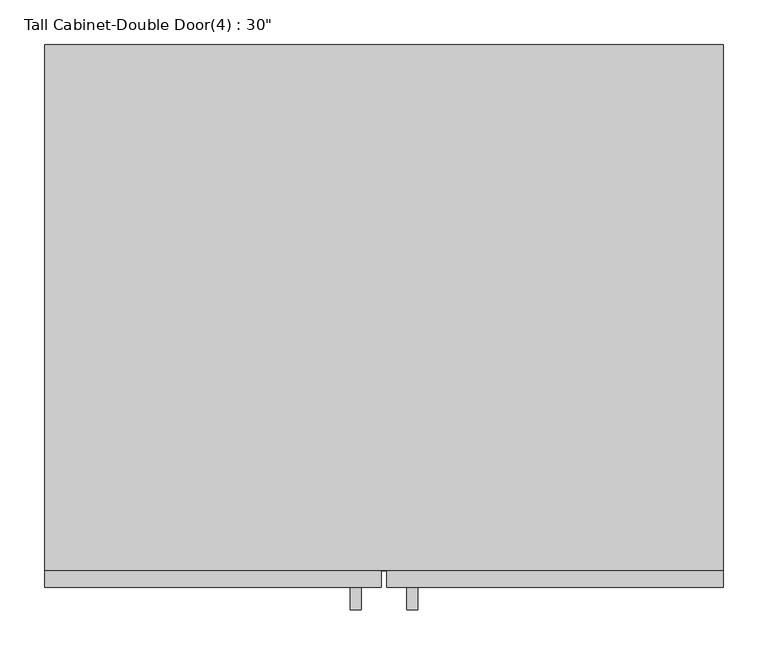
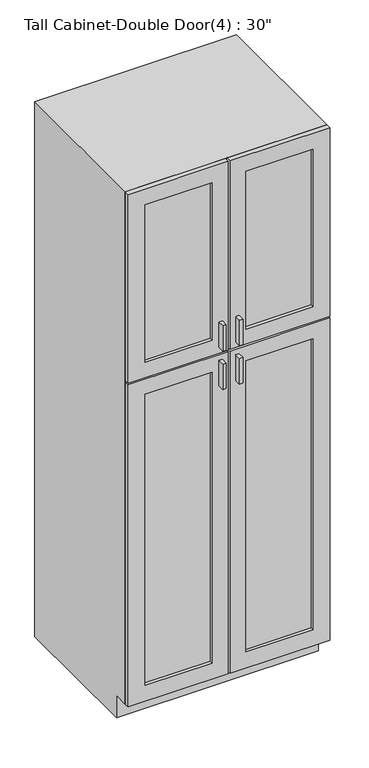
"""IFC4 building model written with IfcOpenShell, lengths in millimetres: furniture geometry."""

from ifc_helpers import new_model, si_unit, frame, origin, place, context, project, spatial, polyline, outline, extrude, faceted_brep, source, transform, mapped, element, save


def furniture_2e4292c0(model_context):
    return source(origin(), model_context, "Body", "SolidModel", [
        faceted_brep([(399.7377049, -590.55, 90.4875), (399.7377049, -590.55, 2133.6), (-362.2622951, -590.55, 2133.6), (-362.2622951, -590.55, 90.4875), (380.6877049, -590.55, 2114.55), (380.6877049, -590.55, 109.5375), (-343.2122951, -590.55, 109.5375), (-343.2122951, -590.55, 2114.55), (-362.2622951, 0.0, 2133.6), (399.7377049, 0.0, 2133.6), (399.7377049, 0.0, 1.5875), (-362.2622951, 0.0, 1.5875), (380.6877049, 0.0, 2114.55), (-343.2122951, 0.0, 2114.55), (-343.2122951, 0.0, 109.5375), (380.6877049, 0.0, 109.5375), (399.7377049, -533.4, 90.4875), (399.7377049, -533.4, 1.5875), (-362.2622951, -533.4, 1.5875), (-362.2622951, -533.4, 90.4875)], [[[0, 1, 2, 3], [4, 5, 6, 7]], [[8, 9, 10, 11], [12, 13, 14, 15]], [[1, 0, 16, 17, 10, 9]], [[2, 1, 9, 8]], [[3, 2, 8, 11, 18, 19]], [[0, 3, 19, 16]], [[5, 4, 12, 15]], [[6, 5, 15, 14]], [[7, 6, 14, 13]], [[4, 7, 13, 12]], [[10, 17, 18, 11]], [[18, 17, 16, 19]]]),
        extrude(outline(polyline([(-6.6622951, -635.0), (-19.1945267, -635.0), (-19.1945267, -609.6), (-6.6622951, -609.6), (-6.6622951, -635.0)])), frame((0.0, 0.0, 1403.5480367), z_axis=(0.0, 0.0, 1.0), x_axis=(1.0, 0.0, 0.0)), (0.0, 0.0, 1.0), 101.6),
        extrude(outline(polyline([(56.6699365, -635.0), (44.1377049, -635.0), (44.1377049, -609.6), (56.6699365, -609.6), (56.6699365, -635.0)])), frame((0.0, 0.0, 1403.5480367), z_axis=(0.0, 0.0, 1.0), x_axis=(1.0, 0.0, 0.0)), (0.0, 0.0, 1.0), 101.6),
        extrude(outline(polyline([(-6.6622951, -635.0), (-19.1945267, -635.0), (-19.1945267, -609.6), (-6.6622951, -609.6), (-6.6622951, -635.0)])), frame((0.0, 0.0, 1251.1480367), z_axis=(0.0, 0.0, 1.0), x_axis=(1.0, 0.0, 0.0)), (0.0, 0.0, 1.0), 101.6),
        extrude(outline(polyline([(56.6699365, -635.0), (44.1377049, -635.0), (44.1377049, -609.6), (56.6699365, -609.6), (56.6699365, -635.0)])), frame((0.0, 0.0, 1251.1480367), z_axis=(0.0, 0.0, 1.0), x_axis=(1.0, 0.0, 0.0)), (0.0, 0.0, 1.0), 101.6),
        extrude(outline(polyline([(-44.7622951, -596.9), (-298.7622951, -596.9), (-298.7622951, -590.55), (-44.7622951, -590.55), (-44.7622951, -596.9)])), frame((0.0, 0.0, 1441.6480367), z_axis=(0.0, 0.0, 1.0), x_axis=(1.0, 0.0, 0.0)), (0.0, 0.0, 1.0), 628.4519633),
        extrude(outline(polyline([(336.2377049, -596.9), (82.2377049, -596.9), (82.2377049, -590.55), (336.2377049, -590.55), (336.2377049, -596.9)])), frame((0.0, 0.0, 1441.6480367), z_axis=(0.0, 0.0, 1.0), x_axis=(1.0, 0.0, 0.0)), (0.0, 0.0, 1.0), 628.4519633),
        extrude(outline(polyline([(-44.7622951, -596.9), (-298.7622951, -596.9), (-298.7622951, -590.55), (-44.7622951, -590.55), (-44.7622951, -596.9)])), frame((0.0, 0.0, 153.9875), z_axis=(0.0, 0.0, 1.0), x_axis=(1.0, 0.0, 0.0)), (0.0, 0.0, 1.0), 1160.6605367),
        extrude(outline(polyline([(336.2377049, -596.9), (82.2377049, -596.9), (82.2377049, -590.55), (336.2377049, -590.55), (336.2377049, -596.9)])), frame((0.0, 0.0, 153.9875), z_axis=(0.0, 0.0, 1.0), x_axis=(1.0, 0.0, 0.0)), (0.0, 0.0, 1.0), 1160.6605367),
        extrude(outline(polyline([(2133.6, 15.5627049), (2133.6, -362.2622951), (1381.3230367, -362.2622951), (1381.3230367, 15.5627049), (2133.6, 15.5627049)]), holes=[polyline([(2070.1, -44.7622951), (1441.6480367, -44.7622951), (1441.6480367, -298.7622951), (2070.1, -298.7622951), (2070.1, -44.7622951)])]), frame((0.0, -609.6, 0.0), z_axis=(0.0, 1.0, 0.0), x_axis=(0.0, 0.0, 1.0)), (0.0, 0.0, 1.0), 19.05),
        extrude(outline(polyline([(2133.6, 21.9127049), (1381.3230367, 21.9127049), (1381.3230367, 399.7377049), (2133.6, 399.7377049), (2133.6, 21.9127049)]), holes=[polyline([(2070.1, 336.2377049), (1441.6480367, 336.2377049), (1441.6480367, 82.2377049), (2070.1, 82.2377049), (2070.1, 336.2377049)])]), frame((0.0, -609.6, 0.0), z_axis=(0.0, 1.0, 0.0), x_axis=(0.0, 0.0, 1.0)), (0.0, 0.0, 1.0), 19.05),
        extrude(outline(polyline([(90.4875, 21.9127049), (90.4875, 399.7377049), (1374.9730367, 399.7377049), (1374.9730367, 21.9127049), (90.4875, 21.9127049)]), holes=[polyline([(1314.6480367, 82.2377049), (1314.6480367, 336.2377049), (153.9875, 336.2377049), (153.9875, 82.2377049), (1314.6480367, 82.2377049)])]), frame((0.0, -609.6, 0.0), z_axis=(0.0, 1.0, 0.0), x_axis=(0.0, 0.0, 1.0)), (0.0, 0.0, 1.0), 19.05),
        extrude(outline(polyline([(90.4875, 15.5627049), (1374.9730367, 15.5627049), (1374.9730367, -362.2622951), (90.4875, -362.2622951), (90.4875, 15.5627049)]), holes=[polyline([(1314.6480367, -44.7622951), (153.9875, -44.7622951), (153.9875, -298.7622951), (1314.6480367, -298.7622951), (1314.6480367, -44.7622951)])]), frame((0.0, -609.6, 0.0), z_axis=(0.0, 1.0, 0.0), x_axis=(0.0, 0.0, 1.0)), (0.0, 0.0, 1.0), 19.05),
        extrude(outline(polyline([(380.6877049, -19.05), (-343.2122951, -19.05), (-343.2122951, 0.0), (380.6877049, 0.0), (380.6877049, -19.05)])), frame((0.0, 0.0, 109.5375), z_axis=(0.0, 0.0, 1.0), x_axis=(1.0, 0.0, 0.0)), (0.0, 0.0, 1.0), 2005.0125),
    ])


if __name__ == "__main__":
    model = new_model("IFC4")
    model_context = context("Model", 3, world=origin())
    ifc_project = project(units=[si_unit("LENGTHUNIT", "METRE", prefix="MILLI")], contexts=[model_context])
    site = spatial("IfcSite", under=ifc_project)
    building = spatial("IfcBuilding", under=site)
    placement = place(None, origin())
    furniture_shape = furniture_2e4292c0(model_context)
    element("IfcFurniture", 1, ObjectType="Tall Cabinet-Double Door(4) : 30\"", at=placement, inside=building, context=model_context, shape_type="MappedRepresentation", body=[
        mapped(furniture_shape, transform((0.0, 0.0, 0.0), x_axis=(1.0, 0.0, 0.0), y_axis=(0.0, 1.0, 0.0), z_axis=(0.0, 0.0, 1.0))),
    ])
    save(model, "model.ifc")

# Revit data of these elements
# Type "Tall Cabinet-Double Door(4) : 30\""
#   Assembly Code = "C1030410"
#   Depth = 2' - 0"
#   Height = 7' - 0"
#   Toe Depth = 0' - 3"
#   Toe Height = 0' - 3 1/2"
#   Width = 2' - 6"
#   Cabinet Material = none
#   Door/Drawer Material = none
#   Handle Material = Cabinets - Handles
#   Panel Material = none
#   Default Elevation = 0
# Element 1 (IfcFurniture, "Tall Cabinet-Double Door(4) : 30\"")
#   Materials on its faces: "Cabinets", "Cabinets - Handles"
# Materials
#   "Cabinets - Handles": class "Metal", colour RGB 57 57 57, transparency 0
#   "Cabinets": colour RGB 249 249 249, transparency 0
